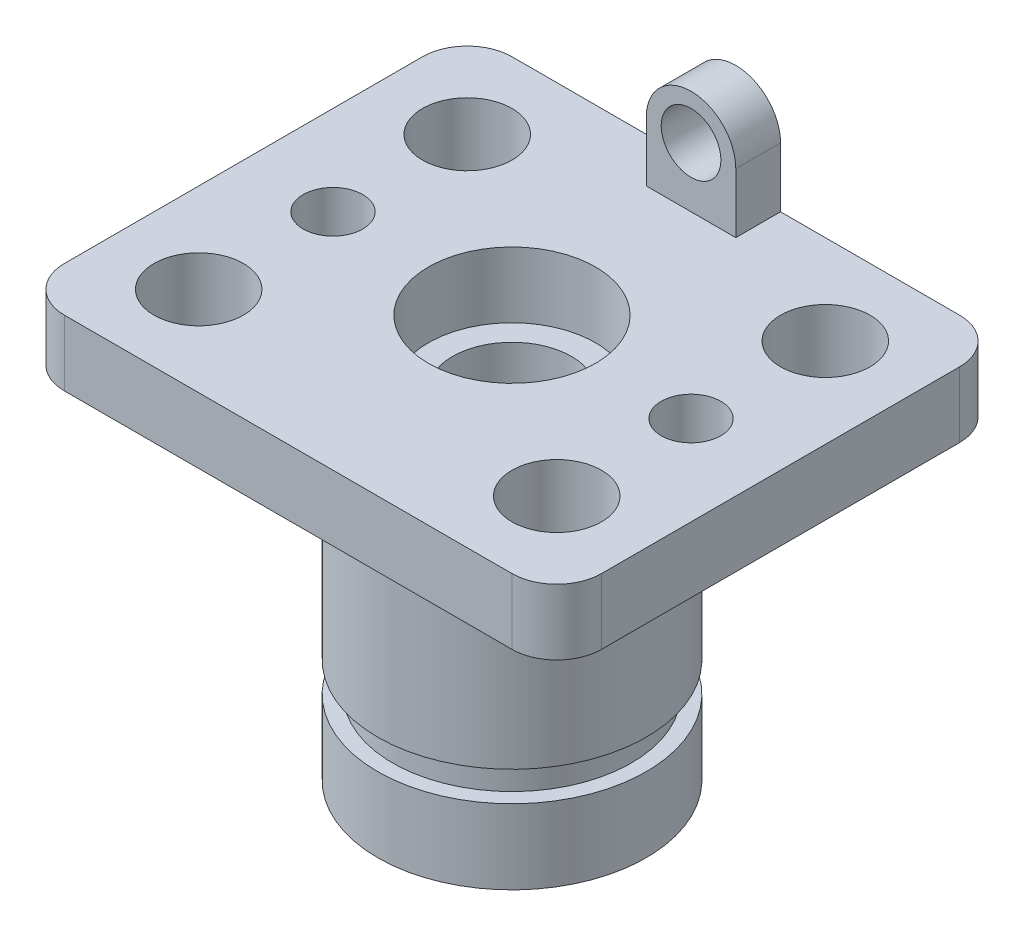
ISO-10303-21;
HEADER;
FILE_DESCRIPTION(('STEP AP214'),'2;1');
FILE_NAME('part.step','',(''),(''),'','','');
FILE_SCHEMA(('AUTOMOTIVE_DESIGN { 1 0 10303 214 1 1 1 1 }'));
ENDSEC;
DATA;
#1=APPLICATION_CONTEXT('core data for automotive mechanical design processes');
#2=APPLICATION_PROTOCOL_DEFINITION('international standard','automotive_design',2000,#1);
#3=PRODUCT_CONTEXT('',#1,'mechanical');
#4=PRODUCT('Part','Part','',(#3));
#5=PRODUCT_RELATED_PRODUCT_CATEGORY('part','',(#4));
#6=PRODUCT_DEFINITION_FORMATION('','',#4);
#7=PRODUCT_DEFINITION_CONTEXT('part definition',#1,'design');
#8=PRODUCT_DEFINITION('design','',#6,#7);
#9=PRODUCT_DEFINITION_SHAPE('','',#8);
#10=(LENGTH_UNIT() NAMED_UNIT(*) SI_UNIT(.MILLI.,.METRE.));
#11=(NAMED_UNIT(*) PLANE_ANGLE_UNIT() SI_UNIT($,.RADIAN.));
#12=(NAMED_UNIT(*) SI_UNIT($,.STERADIAN.) SOLID_ANGLE_UNIT());
#13=UNCERTAINTY_MEASURE_WITH_UNIT(LENGTH_MEASURE(1.E-05),#10,'distance_accuracy_value','');
#14=(GEOMETRIC_REPRESENTATION_CONTEXT(3) GLOBAL_UNCERTAINTY_ASSIGNED_CONTEXT((#13)) GLOBAL_UNIT_ASSIGNED_CONTEXT((#10,
#11,#12)) REPRESENTATION_CONTEXT('',''));
#15=CARTESIAN_POINT('',(0.,0.,0.));
#16=DIRECTION('',(0.,0.,1.));
#17=DIRECTION('',(1.,0.,0.));
#18=AXIS2_PLACEMENT_3D('',#15,#16,#17);
#19=CARTESIAN_POINT('',(-28000.,135000.,0.));
#20=DIRECTION('',(0.,-1.,0.));
#21=DIRECTION('',(0.,0.,-1.));
#22=AXIS2_PLACEMENT_3D('',#19,#20,#21);
#23=PLANE('',#22);
#24=CARTESIAN_POINT('',(0.,135000.,0.));
#25=DIRECTION('',(0.,1.,0.));
#26=DIRECTION('',(0.,0.,1.));
#27=AXIS2_PLACEMENT_3D('',#24,#25,#26);
#28=CIRCLE('',#27,28000.);
#29=CARTESIAN_POINT('',(0.,135000.,28000.));
#30=VERTEX_POINT('',#29);
#31=EDGE_CURVE('E200',#30,#30,#28,.T.);
#32=ORIENTED_EDGE('',*,*,#31,.F.);
#33=EDGE_LOOP('',(#32));
#34=FACE_BOUND('',#33,.T.);
#35=CARTESIAN_POINT('',(-60000.,135000.,45000.));
#36=DIRECTION('',(0.,1.,0.));
#37=DIRECTION('',(0.,0.,1.));
#38=AXIS2_PLACEMENT_3D('',#35,#36,#37);
#39=CIRCLE('',#38,15000.);
#40=CARTESIAN_POINT('',(-60000.,135000.,60000.));
#41=VERTEX_POINT('',#40);
#42=EDGE_CURVE('E195',#41,#41,#39,.T.);
#43=ORIENTED_EDGE('',*,*,#42,.F.);
#44=EDGE_LOOP('',(#43));
#45=FACE_BOUND('',#44,.T.);
#46=CARTESIAN_POINT('',(-60000.,135000.,0.));
#47=DIRECTION('',(0.,1.,0.));
#48=DIRECTION('',(0.,0.,1.));
#49=AXIS2_PLACEMENT_3D('',#46,#47,#48);
#50=CIRCLE('',#49,10000.);
#51=CARTESIAN_POINT('',(-60000.,135000.,10000.));
#52=VERTEX_POINT('',#51);
#53=EDGE_CURVE('E187',#52,#52,#50,.T.);
#54=ORIENTED_EDGE('',*,*,#53,.F.);
#55=EDGE_LOOP('',(#54));
#56=FACE_BOUND('',#55,.T.);
#57=CARTESIAN_POINT('',(-60000.,135000.,-45000.));
#58=DIRECTION('',(0.,1.,0.));
#59=DIRECTION('',(0.,0.,1.));
#60=AXIS2_PLACEMENT_3D('',#57,#58,#59);
#61=CIRCLE('',#60,15000.);
#62=CARTESIAN_POINT('',(-60000.,135000.,-30000.));
#63=VERTEX_POINT('',#62);
#64=EDGE_CURVE('E190',#63,#63,#61,.T.);
#65=ORIENTED_EDGE('',*,*,#64,.F.);
#66=EDGE_LOOP('',(#65));
#67=FACE_BOUND('',#66,.T.);
#68=CARTESIAN_POINT('',(60000.0000000001,135000.,-45000.));
#69=DIRECTION('',(0.,-1.,0.));
#70=DIRECTION('',(0.,0.,-1.));
#71=AXIS2_PLACEMENT_3D('',#68,#69,#70);
#72=CIRCLE('',#71,15000.);
#73=CARTESIAN_POINT('',(60000.0000000001,135000.,-60000.));
#74=VERTEX_POINT('',#73);
#75=EDGE_CURVE('E44',#74,#74,#72,.F.);
#76=ORIENTED_EDGE('',*,*,#75,.F.);
#77=EDGE_LOOP('',(#76));
#78=FACE_BOUND('',#77,.T.);
#79=CARTESIAN_POINT('',(60000.0000000001,135000.,0.));
#80=DIRECTION('',(0.,1.,0.));
#81=DIRECTION('',(0.,0.,1.));
#82=AXIS2_PLACEMENT_3D('',#79,#80,#81);
#83=CIRCLE('',#82,10000.);
#84=CARTESIAN_POINT('',(60000.0000000001,135000.,10000.));
#85=VERTEX_POINT('',#84);
#86=EDGE_CURVE('E172',#85,#85,#83,.T.);
#87=ORIENTED_EDGE('',*,*,#86,.F.);
#88=EDGE_LOOP('',(#87));
#89=FACE_BOUND('',#88,.T.);
#90=CARTESIAN_POINT('',(60000.0000000001,135000.,45000.));
#91=DIRECTION('',(0.,1.,0.));
#92=DIRECTION('',(0.,0.,1.));
#93=AXIS2_PLACEMENT_3D('',#90,#91,#92);
#94=CIRCLE('',#93,15000.);
#95=CARTESIAN_POINT('',(60000.0000000001,135000.,60000.));
#96=VERTEX_POINT('',#95);
#97=EDGE_CURVE('E164',#96,#96,#94,.T.);
#98=ORIENTED_EDGE('',*,*,#97,.F.);
#99=EDGE_LOOP('',(#98));
#100=FACE_BOUND('',#99,.T.);
#101=DIRECTION('',(0.,0.,-1.));
#102=VECTOR('',#101,1.);
#103=CARTESIAN_POINT('',(15000.,135000.,-60000.));
#104=LINE('',#103,#102);
#105=CARTESIAN_POINT('',(15000.,135000.,-60000.));
#106=VERTEX_POINT('',#105);
#107=CARTESIAN_POINT('',(15000.,135000.,-75000.));
#108=VERTEX_POINT('',#107);
#109=EDGE_CURVE('E148',#106,#108,#104,.T.);
#110=ORIENTED_EDGE('',*,*,#109,.F.);
#111=DIRECTION('',(-1.,0.,0.));
#112=VECTOR('',#111,1.);
#113=CARTESIAN_POINT('',(15000.,135000.,-60000.));
#114=LINE('',#113,#112);
#115=CARTESIAN_POINT('',(-15000.,135000.,-60000.));
#116=VERTEX_POINT('',#115);
#117=EDGE_CURVE('E145',#106,#116,#114,.T.);
#118=ORIENTED_EDGE('',*,*,#117,.T.);
#119=DIRECTION('',(0.,0.,-1.));
#120=VECTOR('',#119,1.);
#121=CARTESIAN_POINT('',(-15000.,135000.,-60000.));
#122=LINE('',#121,#120);
#123=CARTESIAN_POINT('',(-15000.,135000.,-75000.));
#124=VERTEX_POINT('',#123);
#125=EDGE_CURVE('E130',#116,#124,#122,.T.);
#126=ORIENTED_EDGE('',*,*,#125,.T.);
#127=DIRECTION('',(-1.,0.,0.));
#128=VECTOR('',#127,1.);
#129=CARTESIAN_POINT('',(-90000.,135000.,-75000.));
#130=LINE('',#129,#128);
#131=CARTESIAN_POINT('',(-75000.,135000.,-75000.));
#132=VERTEX_POINT('',#131);
#133=EDGE_CURVE('E225',#124,#132,#130,.T.);
#134=ORIENTED_EDGE('',*,*,#133,.T.);
#135=CARTESIAN_POINT('',(-75000.,135000.,-60000.));
#136=DIRECTION('',(0.,-1.,0.));
#137=DIRECTION('',(0.,0.,-1.));
#138=AXIS2_PLACEMENT_3D('',#135,#136,#137);
#139=CIRCLE('',#138,15000.);
#140=CARTESIAN_POINT('',(-90000.,135000.,-60000.));
#141=VERTEX_POINT('',#140);
#142=EDGE_CURVE('E271',#132,#141,#139,.F.);
#143=ORIENTED_EDGE('',*,*,#142,.T.);
#144=DIRECTION('',(0.,0.,1.));
#145=VECTOR('',#144,1.);
#146=CARTESIAN_POINT('',(-90000.,135000.,-75000.));
#147=LINE('',#146,#145);
#148=CARTESIAN_POINT('',(-89999.9999999999,135000.,60000.));
#149=VERTEX_POINT('',#148);
#150=EDGE_CURVE('E221',#141,#149,#147,.T.);
#151=ORIENTED_EDGE('',*,*,#150,.T.);
#152=CARTESIAN_POINT('',(-74999.9999999999,135000.,60000.));
#153=DIRECTION('',(0.,-1.,0.));
#154=DIRECTION('',(0.,0.,-1.));
#155=AXIS2_PLACEMENT_3D('',#152,#153,#154);
#156=CIRCLE('',#155,15000.);
#157=CARTESIAN_POINT('',(-74999.9999999999,135000.,75000.));
#158=VERTEX_POINT('',#157);
#159=EDGE_CURVE('E262',#149,#158,#156,.F.);
#160=ORIENTED_EDGE('',*,*,#159,.T.);
#161=DIRECTION('',(1.,0.,0.));
#162=VECTOR('',#161,1.);
#163=CARTESIAN_POINT('',(-89999.9999999999,135000.,75000.));
#164=LINE('',#163,#162);
#165=CARTESIAN_POINT('',(75000.0000000001,135000.,75000.));
#166=VERTEX_POINT('',#165);
#167=EDGE_CURVE('E211',#158,#166,#164,.T.);
#168=ORIENTED_EDGE('',*,*,#167,.T.);
#169=CARTESIAN_POINT('',(75000.0000000001,135000.,60000.));
#170=DIRECTION('',(0.,-1.,0.));
#171=DIRECTION('',(0.,0.,-1.));
#172=AXIS2_PLACEMENT_3D('',#169,#170,#171);
#173=CIRCLE('',#172,15000.);
#174=CARTESIAN_POINT('',(90000.0000000001,135000.,60000.));
#175=VERTEX_POINT('',#174);
#176=EDGE_CURVE('E254',#166,#175,#173,.F.);
#177=ORIENTED_EDGE('',*,*,#176,.T.);
#178=DIRECTION('',(0.,0.,-1.));
#179=VECTOR('',#178,1.);
#180=CARTESIAN_POINT('',(90000.,135000.,-75000.));
#181=LINE('',#180,#179);
#182=CARTESIAN_POINT('',(90000.,135000.,-60000.));
#183=VERTEX_POINT('',#182);
#184=EDGE_CURVE('E220',#175,#183,#181,.T.);
#185=ORIENTED_EDGE('',*,*,#184,.T.);
#186=CARTESIAN_POINT('',(75000.,135000.,-60000.));
#187=DIRECTION('',(0.,-1.,0.));
#188=DIRECTION('',(0.,0.,-1.));
#189=AXIS2_PLACEMENT_3D('',#186,#187,#188);
#190=CIRCLE('',#189,15000.);
#191=CARTESIAN_POINT('',(75000.,135000.,-75000.));
#192=VERTEX_POINT('',#191);
#193=EDGE_CURVE('E282',#183,#192,#190,.F.);
#194=ORIENTED_EDGE('',*,*,#193,.T.);
#195=EDGE_CURVE('E223',#192,#108,#130,.T.);
#196=ORIENTED_EDGE('',*,*,#195,.T.);
#197=EDGE_LOOP('',(#110,#118,#126,#134,#143,#151,#160,#168,#177,#185,#194,#196));
#198=FACE_BOUND('',#197,.T.);
#199=ADVANCED_FACE('F41',(#34,#45,#56,#67,#78,#89,#100,#198),#23,.F.);
#200=CARTESIAN_POINT('',(0.,0.,0.));
#201=DIRECTION('',(0.,-1.,0.));
#202=DIRECTION('',(0.,0.,-1.));
#203=AXIS2_PLACEMENT_3D('',#200,#201,#202);
#204=CYLINDRICAL_SURFACE('',#203,20000.);
#205=CARTESIAN_POINT('',(0.,0.,0.));
#206=DIRECTION('',(0.,-1.,0.));
#207=DIRECTION('',(0.,0.,-1.));
#208=AXIS2_PLACEMENT_3D('',#205,#206,#207);
#209=CIRCLE('',#208,20000.);
#210=CARTESIAN_POINT('',(0.,0.,-20000.));
#211=VERTEX_POINT('',#210);
#212=EDGE_CURVE('E242',#211,#211,#209,.T.);
#213=ORIENTED_EDGE('',*,*,#212,.T.);
#214=EDGE_LOOP('',(#213));
#215=FACE_BOUND('',#214,.T.);
#216=CARTESIAN_POINT('',(0.,113000.,0.));
#217=DIRECTION('',(0.,1.,0.));
#218=DIRECTION('',(0.,0.,1.));
#219=AXIS2_PLACEMENT_3D('',#216,#217,#218);
#220=CIRCLE('',#219,20000.);
#221=CARTESIAN_POINT('',(0.,113000.,20000.));
#222=VERTEX_POINT('',#221);
#223=EDGE_CURVE('E201',#222,#222,#220,.F.);
#224=ORIENTED_EDGE('',*,*,#223,.F.);
#225=EDGE_LOOP('',(#224));
#226=FACE_BOUND('',#225,.T.);
#227=ADVANCED_FACE('F331',(#215,#226),#204,.F.);
#228=CARTESIAN_POINT('',(0.,0.,0.));
#229=DIRECTION('',(0.,-1.,0.));
#230=DIRECTION('',(0.,0.,-1.));
#231=AXIS2_PLACEMENT_3D('',#228,#229,#230);
#232=CYLINDRICAL_SURFACE('',#231,45000.);
#233=CARTESIAN_POINT('',(0.,35000.,0.));
#234=DIRECTION('',(0.,-1.,0.));
#235=DIRECTION('',(0.,0.,-1.));
#236=AXIS2_PLACEMENT_3D('',#233,#234,#235);
#237=CIRCLE('',#236,45000.);
#238=CARTESIAN_POINT('',(0.,35000.,-45000.));
#239=VERTEX_POINT('',#238);
#240=EDGE_CURVE('E241',#239,#239,#237,.T.);
#241=ORIENTED_EDGE('',*,*,#240,.F.);
#242=EDGE_LOOP('',(#241));
#243=FACE_BOUND('',#242,.T.);
#244=CARTESIAN_POINT('',(0.,113000.,0.));
#245=DIRECTION('',(0.,1.,0.));
#246=DIRECTION('',(0.,0.,1.));
#247=AXIS2_PLACEMENT_3D('',#244,#245,#246);
#248=CIRCLE('',#247,45000.);
#249=CARTESIAN_POINT('',(0.,113000.,45000.));
#250=VERTEX_POINT('',#249);
#251=EDGE_CURVE('E250',#250,#250,#248,.T.);
#252=ORIENTED_EDGE('',*,*,#251,.F.);
#253=EDGE_LOOP('',(#252));
#254=FACE_BOUND('',#253,.T.);
#255=ADVANCED_FACE('F345',(#243,#254),#232,.T.);
#256=CARTESIAN_POINT('',(-45000.,-2.36390366877063E-12,0.));
#257=DIRECTION('',(0.,1.,0.));
#258=DIRECTION('',(0.,0.,1.));
#259=AXIS2_PLACEMENT_3D('',#256,#257,#258);
#260=PLANE('',#259);
#261=ORIENTED_EDGE('',*,*,#212,.F.);
#262=EDGE_LOOP('',(#261));
#263=FACE_BOUND('',#262,.T.);
#264=CARTESIAN_POINT('',(0.,-4.72780733754125E-12,0.));
#265=DIRECTION('',(0.,-1.,0.));
#266=DIRECTION('',(0.,0.,-1.));
#267=AXIS2_PLACEMENT_3D('',#264,#265,#266);
#268=CIRCLE('',#267,45000.);
#269=CARTESIAN_POINT('',(0.,-4.72780733754125E-12,-45000.));
#270=VERTEX_POINT('',#269);
#271=EDGE_CURVE('E217',#270,#270,#268,.T.);
#272=ORIENTED_EDGE('',*,*,#271,.T.);
#273=EDGE_LOOP('',(#272));
#274=FACE_BOUND('',#273,.T.);
#275=ADVANCED_FACE('F352',(#263,#274),#260,.F.);
#276=CARTESIAN_POINT('',(-45000.,35000.,0.));
#277=DIRECTION('',(0.,1.,0.));
#278=DIRECTION('',(0.,0.,1.));
#279=AXIS2_PLACEMENT_3D('',#276,#277,#278);
#280=PLANE('',#279);
#281=CARTESIAN_POINT('',(0.,35000.,0.));
#282=DIRECTION('',(0.,-1.,0.));
#283=DIRECTION('',(0.,0.,-1.));
#284=AXIS2_PLACEMENT_3D('',#281,#282,#283);
#285=CIRCLE('',#284,40000.);
#286=CARTESIAN_POINT('',(0.,35000.,-40000.));
#287=VERTEX_POINT('',#286);
#288=EDGE_CURVE('E238',#287,#287,#285,.T.);
#289=ORIENTED_EDGE('',*,*,#288,.F.);
#290=EDGE_LOOP('',(#289));
#291=FACE_BOUND('',#290,.T.);
#292=ORIENTED_EDGE('',*,*,#240,.T.);
#293=EDGE_LOOP('',(#292));
#294=FACE_BOUND('',#293,.T.);
#295=ADVANCED_FACE('F354',(#291,#294),#280,.F.);
#296=CARTESIAN_POINT('',(0.,0.,0.));
#297=DIRECTION('',(0.,-1.,0.));
#298=DIRECTION('',(0.,0.,-1.));
#299=AXIS2_PLACEMENT_3D('',#296,#297,#298);
#300=CYLINDRICAL_SURFACE('',#299,40000.);
#301=CARTESIAN_POINT('',(0.,25000.,0.));
#302=DIRECTION('',(0.,-1.,0.));
#303=DIRECTION('',(0.,0.,-1.));
#304=AXIS2_PLACEMENT_3D('',#301,#302,#303);
#305=CIRCLE('',#304,40000.);
#306=CARTESIAN_POINT('',(0.,25000.,-40000.));
#307=VERTEX_POINT('',#306);
#308=EDGE_CURVE('E232',#307,#307,#305,.T.);
#309=ORIENTED_EDGE('',*,*,#308,.F.);
#310=EDGE_LOOP('',(#309));
#311=FACE_BOUND('',#310,.T.);
#312=ORIENTED_EDGE('',*,*,#288,.T.);
#313=EDGE_LOOP('',(#312));
#314=FACE_BOUND('',#313,.T.);
#315=ADVANCED_FACE('F420',(#311,#314),#300,.T.);
#316=CARTESIAN_POINT('',(-40000.,25000.,0.));
#317=DIRECTION('',(0.,-1.,0.));
#318=DIRECTION('',(0.,0.,-1.));
#319=AXIS2_PLACEMENT_3D('',#316,#317,#318);
#320=PLANE('',#319);
#321=CARTESIAN_POINT('',(0.,25000.,0.));
#322=DIRECTION('',(0.,-1.,0.));
#323=DIRECTION('',(0.,0.,-1.));
#324=AXIS2_PLACEMENT_3D('',#321,#322,#323);
#325=CIRCLE('',#324,45000.);
#326=CARTESIAN_POINT('',(0.,25000.,-45000.));
#327=VERTEX_POINT('',#326);
#328=EDGE_CURVE('E235',#327,#327,#325,.T.);
#329=ORIENTED_EDGE('',*,*,#328,.F.);
#330=EDGE_LOOP('',(#329));
#331=FACE_BOUND('',#330,.T.);
#332=ORIENTED_EDGE('',*,*,#308,.T.);
#333=EDGE_LOOP('',(#332));
#334=FACE_BOUND('',#333,.T.);
#335=ADVANCED_FACE('F395',(#331,#334),#320,.F.);
#336=CARTESIAN_POINT('',(0.,0.,0.));
#337=DIRECTION('',(0.,-1.,0.));
#338=DIRECTION('',(0.,0.,-1.));
#339=AXIS2_PLACEMENT_3D('',#336,#337,#338);
#340=CYLINDRICAL_SURFACE('',#339,45000.);
#341=ORIENTED_EDGE('',*,*,#271,.F.);
#342=EDGE_LOOP('',(#341));
#343=FACE_BOUND('',#342,.T.);
#344=ORIENTED_EDGE('',*,*,#328,.T.);
#345=EDGE_LOOP('',(#344));
#346=FACE_BOUND('',#345,.T.);
#347=ADVANCED_FACE('F383',(#343,#346),#340,.T.);
#348=CARTESIAN_POINT('',(0.,113000.,0.));
#349=DIRECTION('',(0.,1.,0.));
#350=DIRECTION('',(0.,0.,1.));
#351=AXIS2_PLACEMENT_3D('',#348,#349,#350);
#352=PLANE('',#351);
#353=CARTESIAN_POINT('',(60000.0000000001,113000.,45000.));
#354=DIRECTION('',(0.,1.,0.));
#355=DIRECTION('',(0.,0.,1.));
#356=AXIS2_PLACEMENT_3D('',#353,#354,#355);
#357=CIRCLE('',#356,15000.);
#358=CARTESIAN_POINT('',(60000.0000000001,113000.,60000.));
#359=VERTEX_POINT('',#358);
#360=EDGE_CURVE('E171',#359,#359,#357,.F.);
#361=ORIENTED_EDGE('',*,*,#360,.F.);
#362=EDGE_LOOP('',(#361));
#363=FACE_BOUND('',#362,.T.);
#364=CARTESIAN_POINT('',(60000.0000000001,113000.,0.));
#365=DIRECTION('',(0.,1.,0.));
#366=DIRECTION('',(0.,0.,1.));
#367=AXIS2_PLACEMENT_3D('',#364,#365,#366);
#368=CIRCLE('',#367,10000.);
#369=CARTESIAN_POINT('',(60000.0000000001,113000.,10000.));
#370=VERTEX_POINT('',#369);
#371=EDGE_CURVE('E180',#370,#370,#368,.F.);
#372=ORIENTED_EDGE('',*,*,#371,.F.);
#373=EDGE_LOOP('',(#372));
#374=FACE_BOUND('',#373,.T.);
#375=CARTESIAN_POINT('',(60000.0000000001,113000.,-45000.));
#376=DIRECTION('',(0.,1.,0.));
#377=DIRECTION('',(0.,0.,1.));
#378=AXIS2_PLACEMENT_3D('',#375,#376,#377);
#379=CIRCLE('',#378,15000.);
#380=CARTESIAN_POINT('',(60000.0000000001,113000.,-60000.));
#381=VERTEX_POINT('',#380);
#382=EDGE_CURVE('E179',#381,#381,#379,.F.);
#383=ORIENTED_EDGE('',*,*,#382,.F.);
#384=EDGE_LOOP('',(#383));
#385=FACE_BOUND('',#384,.T.);
#386=CARTESIAN_POINT('',(-60000.,113000.,-45000.));
#387=DIRECTION('',(0.,1.,0.));
#388=DIRECTION('',(0.,0.,1.));
#389=AXIS2_PLACEMENT_3D('',#386,#387,#388);
#390=CIRCLE('',#389,15000.);
#391=CARTESIAN_POINT('',(-60000.,113000.,-30000.));
#392=VERTEX_POINT('',#391);
#393=EDGE_CURVE('E182',#392,#392,#390,.T.);
#394=ORIENTED_EDGE('',*,*,#393,.T.);
#395=EDGE_LOOP('',(#394));
#396=FACE_BOUND('',#395,.T.);
#397=CARTESIAN_POINT('',(-60000.,113000.,0.));
#398=DIRECTION('',(0.,1.,0.));
#399=DIRECTION('',(0.,0.,1.));
#400=AXIS2_PLACEMENT_3D('',#397,#398,#399);
#401=CIRCLE('',#400,10000.);
#402=CARTESIAN_POINT('',(-60000.,113000.,10000.));
#403=VERTEX_POINT('',#402);
#404=EDGE_CURVE('E188',#403,#403,#401,.T.);
#405=ORIENTED_EDGE('',*,*,#404,.T.);
#406=EDGE_LOOP('',(#405));
#407=FACE_BOUND('',#406,.T.);
#408=CARTESIAN_POINT('',(-60000.,113000.,45000.));
#409=DIRECTION('',(0.,1.,0.));
#410=DIRECTION('',(0.,0.,1.));
#411=AXIS2_PLACEMENT_3D('',#408,#409,#410);
#412=CIRCLE('',#411,15000.);
#413=CARTESIAN_POINT('',(-60000.,113000.,60000.));
#414=VERTEX_POINT('',#413);
#415=EDGE_CURVE('E198',#414,#414,#412,.T.);
#416=ORIENTED_EDGE('',*,*,#415,.T.);
#417=EDGE_LOOP('',(#416));
#418=FACE_BOUND('',#417,.T.);
#419=ORIENTED_EDGE('',*,*,#251,.T.);
#420=EDGE_LOOP('',(#419));
#421=FACE_BOUND('',#420,.T.);
#422=DIRECTION('',(-1.,0.,0.));
#423=VECTOR('',#422,1.);
#424=CARTESIAN_POINT('',(-90000.,113000.,-75000.));
#425=LINE('',#424,#423);
#426=CARTESIAN_POINT('',(75000.,113000.,-75000.));
#427=VERTEX_POINT('',#426);
#428=CARTESIAN_POINT('',(-75000.,113000.,-75000.));
#429=VERTEX_POINT('',#428);
#430=EDGE_CURVE('E214',#427,#429,#425,.T.);
#431=ORIENTED_EDGE('',*,*,#430,.F.);
#432=CARTESIAN_POINT('',(75000.,113000.,-60000.));
#433=DIRECTION('',(0.,1.,0.));
#434=DIRECTION('',(0.,0.,1.));
#435=AXIS2_PLACEMENT_3D('',#432,#433,#434);
#436=CIRCLE('',#435,15000.);
#437=CARTESIAN_POINT('',(90000.,113000.,-60000.));
#438=VERTEX_POINT('',#437);
#439=EDGE_CURVE('E11',#427,#438,#436,.F.);
#440=ORIENTED_EDGE('',*,*,#439,.T.);
#441=DIRECTION('',(0.,0.,-1.));
#442=VECTOR('',#441,1.);
#443=CARTESIAN_POINT('',(90000.,113000.,-75000.));
#444=LINE('',#443,#442);
#445=CARTESIAN_POINT('',(90000.0000000001,113000.,60000.));
#446=VERTEX_POINT('',#445);
#447=EDGE_CURVE('E206',#446,#438,#444,.T.);
#448=ORIENTED_EDGE('',*,*,#447,.F.);
#449=CARTESIAN_POINT('',(75000.0000000001,113000.,60000.));
#450=DIRECTION('',(0.,1.,0.));
#451=DIRECTION('',(0.,0.,1.));
#452=AXIS2_PLACEMENT_3D('',#449,#450,#451);
#453=CIRCLE('',#452,15000.);
#454=CARTESIAN_POINT('',(75000.0000000001,113000.,75000.));
#455=VERTEX_POINT('',#454);
#456=EDGE_CURVE('E256',#446,#455,#453,.F.);
#457=ORIENTED_EDGE('',*,*,#456,.T.);
#458=DIRECTION('',(1.,0.,0.));
#459=VECTOR('',#458,1.);
#460=CARTESIAN_POINT('',(-89999.9999999999,113000.,75000.));
#461=LINE('',#460,#459);
#462=CARTESIAN_POINT('',(-74999.9999999999,113000.,75000.));
#463=VERTEX_POINT('',#462);
#464=EDGE_CURVE('E218',#463,#455,#461,.T.);
#465=ORIENTED_EDGE('',*,*,#464,.F.);
#466=CARTESIAN_POINT('',(-74999.9999999999,113000.,60000.));
#467=DIRECTION('',(0.,1.,0.));
#468=DIRECTION('',(0.,0.,1.));
#469=AXIS2_PLACEMENT_3D('',#466,#467,#468);
#470=CIRCLE('',#469,15000.);
#471=CARTESIAN_POINT('',(-89999.9999999999,113000.,60000.));
#472=VERTEX_POINT('',#471);
#473=EDGE_CURVE('E270',#463,#472,#470,.F.);
#474=ORIENTED_EDGE('',*,*,#473,.T.);
#475=DIRECTION('',(0.,0.,1.));
#476=VECTOR('',#475,1.);
#477=CARTESIAN_POINT('',(-90000.,113000.,-75000.));
#478=LINE('',#477,#476);
#479=CARTESIAN_POINT('',(-90000.,113000.,-60000.));
#480=VERTEX_POINT('',#479);
#481=EDGE_CURVE('E213',#480,#472,#478,.T.);
#482=ORIENTED_EDGE('',*,*,#481,.F.);
#483=CARTESIAN_POINT('',(-75000.,113000.,-60000.));
#484=DIRECTION('',(0.,1.,0.));
#485=DIRECTION('',(0.,0.,1.));
#486=AXIS2_PLACEMENT_3D('',#483,#484,#485);
#487=CIRCLE('',#486,15000.);
#488=EDGE_CURVE('E276',#480,#429,#487,.F.);
#489=ORIENTED_EDGE('',*,*,#488,.T.);
#490=EDGE_LOOP('',(#431,#440,#448,#457,#465,#474,#482,#489));
#491=FACE_BOUND('',#490,.T.);
#492=ADVANCED_FACE('F291',(#363,#374,#385,#396,#407,#418,#421,#491),#352,.F.);
#493=CARTESIAN_POINT('',(-90000.,113000.,-75000.));
#494=DIRECTION('',(0.,0.,-1.));
#495=DIRECTION('',(-1.,0.,0.));
#496=AXIS2_PLACEMENT_3D('',#493,#494,#495);
#497=PLANE('',#496);
#498=CARTESIAN_POINT('',(0.,155000.,-75000.));
#499=DIRECTION('',(0.,0.,-1.));
#500=DIRECTION('',(-1.,0.,0.));
#501=AXIS2_PLACEMENT_3D('',#498,#499,#500);
#502=CIRCLE('',#501,10000.);
#503=CARTESIAN_POINT('',(-10000.,155000.,-75000.));
#504=VERTEX_POINT('',#503);
#505=EDGE_CURVE('E605',#504,#504,#502,.T.);
#506=ORIENTED_EDGE('',*,*,#505,.F.);
#507=EDGE_LOOP('',(#506));
#508=FACE_BOUND('',#507,.T.);
#509=ORIENTED_EDGE('',*,*,#195,.F.);
#510=DIRECTION('',(0.,1.,0.));
#511=VECTOR('',#510,1.);
#512=CARTESIAN_POINT('',(75000.,113000.,-75000.));
#513=LINE('',#512,#511);
#514=EDGE_CURVE('E49',#192,#427,#513,.F.);
#515=ORIENTED_EDGE('',*,*,#514,.T.);
#516=ORIENTED_EDGE('',*,*,#430,.T.);
#517=DIRECTION('',(0.,1.,0.));
#518=VECTOR('',#517,1.);
#519=CARTESIAN_POINT('',(-75000.,113000.,-75000.));
#520=LINE('',#519,#518);
#521=EDGE_CURVE('E266',#429,#132,#520,.T.);
#522=ORIENTED_EDGE('',*,*,#521,.T.);
#523=ORIENTED_EDGE('',*,*,#133,.F.);
#524=DIRECTION('',(0.,1.,0.));
#525=VECTOR('',#524,1.);
#526=CARTESIAN_POINT('',(-15000.,135000.,-75000.));
#527=LINE('',#526,#525);
#528=CARTESIAN_POINT('',(-15000.,155000.,-75000.));
#529=VERTEX_POINT('',#528);
#530=EDGE_CURVE('E60',#124,#529,#527,.T.);
#531=ORIENTED_EDGE('',*,*,#530,.T.);
#532=CARTESIAN_POINT('',(0.,155000.,-75000.));
#533=DIRECTION('',(0.,0.,-1.));
#534=DIRECTION('',(-1.,0.,0.));
#535=AXIS2_PLACEMENT_3D('',#532,#533,#534);
#536=CIRCLE('',#535,15000.);
#537=CARTESIAN_POINT('',(15000.,155000.,-75000.));
#538=VERTEX_POINT('',#537);
#539=EDGE_CURVE('E152',#529,#538,#536,.T.);
#540=ORIENTED_EDGE('',*,*,#539,.T.);
#541=DIRECTION('',(0.,-1.,0.));
#542=VECTOR('',#541,1.);
#543=CARTESIAN_POINT('',(15000.,155000.,-75000.));
#544=LINE('',#543,#542);
#545=EDGE_CURVE('E147',#538,#108,#544,.T.);
#546=ORIENTED_EDGE('',*,*,#545,.T.);
#547=EDGE_LOOP('',(#509,#515,#516,#522,#523,#531,#540,#546));
#548=FACE_BOUND('',#547,.T.);
#549=ADVANCED_FACE('F288',(#508,#548),#497,.T.);
#550=CARTESIAN_POINT('',(-90000.,113000.,-75000.));
#551=DIRECTION('',(-1.,0.,0.));
#552=DIRECTION('',(0.,0.,1.));
#553=AXIS2_PLACEMENT_3D('',#550,#551,#552);
#554=PLANE('',#553);
#555=ORIENTED_EDGE('',*,*,#150,.F.);
#556=DIRECTION('',(0.,1.,0.));
#557=VECTOR('',#556,1.);
#558=CARTESIAN_POINT('',(-90000.,113000.,-60000.));
#559=LINE('',#558,#557);
#560=EDGE_CURVE('E273',#141,#480,#559,.F.);
#561=ORIENTED_EDGE('',*,*,#560,.T.);
#562=ORIENTED_EDGE('',*,*,#481,.T.);
#563=DIRECTION('',(0.,1.,0.));
#564=VECTOR('',#563,1.);
#565=CARTESIAN_POINT('',(-89999.9999999999,113000.,60000.));
#566=LINE('',#565,#564);
#567=EDGE_CURVE('E257',#472,#149,#566,.T.);
#568=ORIENTED_EDGE('',*,*,#567,.T.);
#569=EDGE_LOOP('',(#555,#561,#562,#568));
#570=FACE_BOUND('',#569,.T.);
#571=ADVANCED_FACE('F312',(#570),#554,.T.);
#572=CARTESIAN_POINT('',(-89999.9999999999,113000.,75000.));
#573=DIRECTION('',(0.,0.,1.));
#574=DIRECTION('',(1.,0.,0.));
#575=AXIS2_PLACEMENT_3D('',#572,#573,#574);
#576=PLANE('',#575);
#577=ORIENTED_EDGE('',*,*,#167,.F.);
#578=DIRECTION('',(0.,1.,0.));
#579=VECTOR('',#578,1.);
#580=CARTESIAN_POINT('',(-74999.9999999999,113000.,75000.));
#581=LINE('',#580,#579);
#582=EDGE_CURVE('E261',#158,#463,#581,.F.);
#583=ORIENTED_EDGE('',*,*,#582,.T.);
#584=ORIENTED_EDGE('',*,*,#464,.T.);
#585=DIRECTION('',(0.,1.,0.));
#586=VECTOR('',#585,1.);
#587=CARTESIAN_POINT('',(75000.0000000001,113000.,75000.));
#588=LINE('',#587,#586);
#589=EDGE_CURVE('E249',#455,#166,#588,.T.);
#590=ORIENTED_EDGE('',*,*,#589,.T.);
#591=EDGE_LOOP('',(#577,#583,#584,#590));
#592=FACE_BOUND('',#591,.T.);
#593=ADVANCED_FACE('F324',(#592),#576,.T.);
#594=CARTESIAN_POINT('',(90000.,113000.,-75000.));
#595=DIRECTION('',(1.,0.,0.));
#596=DIRECTION('',(0.,0.,-1.));
#597=AXIS2_PLACEMENT_3D('',#594,#595,#596);
#598=PLANE('',#597);
#599=ORIENTED_EDGE('',*,*,#447,.T.);
#600=DIRECTION('',(0.,1.,0.));
#601=VECTOR('',#600,1.);
#602=CARTESIAN_POINT('',(90000.,113000.,-60000.));
#603=LINE('',#602,#601);
#604=EDGE_CURVE('E277',#438,#183,#603,.T.);
#605=ORIENTED_EDGE('',*,*,#604,.T.);
#606=ORIENTED_EDGE('',*,*,#184,.F.);
#607=DIRECTION('',(0.,1.,0.));
#608=VECTOR('',#607,1.);
#609=CARTESIAN_POINT('',(90000.0000000001,113000.,60000.));
#610=LINE('',#609,#608);
#611=EDGE_CURVE('E253',#175,#446,#610,.F.);
#612=ORIENTED_EDGE('',*,*,#611,.T.);
#613=EDGE_LOOP('',(#599,#605,#606,#612));
#614=FACE_BOUND('',#613,.T.);
#615=ADVANCED_FACE('F298',(#614),#598,.T.);
#616=CARTESIAN_POINT('',(0.,113000.,0.));
#617=DIRECTION('',(0.,1.,0.));
#618=DIRECTION('',(0.,0.,1.));
#619=AXIS2_PLACEMENT_3D('',#616,#617,#618);
#620=PLANE('',#619);
#621=CARTESIAN_POINT('',(0.,113000.,0.));
#622=DIRECTION('',(0.,1.,0.));
#623=DIRECTION('',(0.,0.,1.));
#624=AXIS2_PLACEMENT_3D('',#621,#622,#623);
#625=CIRCLE('',#624,28000.);
#626=CARTESIAN_POINT('',(0.,113000.,28000.));
#627=VERTEX_POINT('',#626);
#628=EDGE_CURVE('E205',#627,#627,#625,.T.);
#629=ORIENTED_EDGE('',*,*,#628,.T.);
#630=EDGE_LOOP('',(#629));
#631=FACE_BOUND('',#630,.T.);
#632=ORIENTED_EDGE('',*,*,#223,.T.);
#633=EDGE_LOOP('',(#632));
#634=FACE_BOUND('',#633,.T.);
#635=ADVANCED_FACE('F330',(#631,#634),#620,.T.);
#636=CARTESIAN_POINT('',(0.,113000.,0.));
#637=DIRECTION('',(0.,1.,0.));
#638=DIRECTION('',(0.,0.,1.));
#639=AXIS2_PLACEMENT_3D('',#636,#637,#638);
#640=CYLINDRICAL_SURFACE('',#639,28000.);
#641=ORIENTED_EDGE('',*,*,#628,.F.);
#642=EDGE_LOOP('',(#641));
#643=FACE_BOUND('',#642,.T.);
#644=ORIENTED_EDGE('',*,*,#31,.T.);
#645=EDGE_LOOP('',(#644));
#646=FACE_BOUND('',#645,.T.);
#647=ADVANCED_FACE('F357',(#643,#646),#640,.F.);
#648=CARTESIAN_POINT('',(75000.0000000001,113000.,60000.));
#649=DIRECTION('',(0.,1.,0.));
#650=DIRECTION('',(0.,0.,1.));
#651=AXIS2_PLACEMENT_3D('',#648,#649,#650);
#652=CYLINDRICAL_SURFACE('',#651,15000.);
#653=ORIENTED_EDGE('',*,*,#456,.F.);
#654=ORIENTED_EDGE('',*,*,#611,.F.);
#655=ORIENTED_EDGE('',*,*,#176,.F.);
#656=ORIENTED_EDGE('',*,*,#589,.F.);
#657=EDGE_LOOP('',(#653,#654,#655,#656));
#658=FACE_BOUND('',#657,.T.);
#659=ADVANCED_FACE('F297',(#658),#652,.T.);
#660=CARTESIAN_POINT('',(-74999.9999999999,113000.,60000.));
#661=DIRECTION('',(0.,1.,0.));
#662=DIRECTION('',(0.,0.,1.));
#663=AXIS2_PLACEMENT_3D('',#660,#661,#662);
#664=CYLINDRICAL_SURFACE('',#663,15000.);
#665=ORIENTED_EDGE('',*,*,#473,.F.);
#666=ORIENTED_EDGE('',*,*,#582,.F.);
#667=ORIENTED_EDGE('',*,*,#159,.F.);
#668=ORIENTED_EDGE('',*,*,#567,.F.);
#669=EDGE_LOOP('',(#665,#666,#667,#668));
#670=FACE_BOUND('',#669,.T.);
#671=ADVANCED_FACE('F307',(#670),#664,.T.);
#672=CARTESIAN_POINT('',(-75000.,113000.,-60000.));
#673=DIRECTION('',(0.,1.,0.));
#674=DIRECTION('',(0.,0.,1.));
#675=AXIS2_PLACEMENT_3D('',#672,#673,#674);
#676=CYLINDRICAL_SURFACE('',#675,15000.);
#677=ORIENTED_EDGE('',*,*,#488,.F.);
#678=ORIENTED_EDGE('',*,*,#560,.F.);
#679=ORIENTED_EDGE('',*,*,#142,.F.);
#680=ORIENTED_EDGE('',*,*,#521,.F.);
#681=EDGE_LOOP('',(#677,#678,#679,#680));
#682=FACE_BOUND('',#681,.T.);
#683=ADVANCED_FACE('F319',(#682),#676,.T.);
#684=CARTESIAN_POINT('',(75000.,113000.,-60000.));
#685=DIRECTION('',(0.,1.,0.));
#686=DIRECTION('',(0.,0.,1.));
#687=AXIS2_PLACEMENT_3D('',#684,#685,#686);
#688=CYLINDRICAL_SURFACE('',#687,15000.);
#689=ORIENTED_EDGE('',*,*,#439,.F.);
#690=ORIENTED_EDGE('',*,*,#514,.F.);
#691=ORIENTED_EDGE('',*,*,#193,.F.);
#692=ORIENTED_EDGE('',*,*,#604,.F.);
#693=EDGE_LOOP('',(#689,#690,#691,#692));
#694=FACE_BOUND('',#693,.T.);
#695=ADVANCED_FACE('F43',(#694),#688,.T.);
#696=CARTESIAN_POINT('',(-60000.,113000.,45000.));
#697=DIRECTION('',(0.,1.,0.));
#698=DIRECTION('',(0.,0.,1.));
#699=AXIS2_PLACEMENT_3D('',#696,#697,#698);
#700=CYLINDRICAL_SURFACE('',#699,15000.);
#701=ORIENTED_EDGE('',*,*,#415,.F.);
#702=EDGE_LOOP('',(#701));
#703=FACE_BOUND('',#702,.T.);
#704=ORIENTED_EDGE('',*,*,#42,.T.);
#705=EDGE_LOOP('',(#704));
#706=FACE_BOUND('',#705,.T.);
#707=ADVANCED_FACE('F365',(#703,#706),#700,.F.);
#708=CARTESIAN_POINT('',(-60000.,113000.,0.));
#709=DIRECTION('',(0.,1.,0.));
#710=DIRECTION('',(0.,0.,1.));
#711=AXIS2_PLACEMENT_3D('',#708,#709,#710);
#712=CYLINDRICAL_SURFACE('',#711,10000.);
#713=ORIENTED_EDGE('',*,*,#404,.F.);
#714=EDGE_LOOP('',(#713));
#715=FACE_BOUND('',#714,.T.);
#716=ORIENTED_EDGE('',*,*,#53,.T.);
#717=EDGE_LOOP('',(#716));
#718=FACE_BOUND('',#717,.T.);
#719=ADVANCED_FACE('F366',(#715,#718),#712,.F.);
#720=CARTESIAN_POINT('',(-60000.,113000.,-45000.));
#721=DIRECTION('',(0.,1.,0.));
#722=DIRECTION('',(0.,0.,1.));
#723=AXIS2_PLACEMENT_3D('',#720,#721,#722);
#724=CYLINDRICAL_SURFACE('',#723,15000.);
#725=ORIENTED_EDGE('',*,*,#393,.F.);
#726=EDGE_LOOP('',(#725));
#727=FACE_BOUND('',#726,.T.);
#728=ORIENTED_EDGE('',*,*,#64,.T.);
#729=EDGE_LOOP('',(#728));
#730=FACE_BOUND('',#729,.T.);
#731=ADVANCED_FACE('F375',(#727,#730),#724,.F.);
#732=CARTESIAN_POINT('',(60000.0000000001,135000.000012,-45000.));
#733=DIRECTION('',(0.,-1.,0.));
#734=DIRECTION('',(0.,0.,-1.));
#735=AXIS2_PLACEMENT_3D('',#732,#733,#734);
#736=CYLINDRICAL_SURFACE('',#735,15000.);
#737=CARTESIAN_POINT('',(60000.0000000001,113000.,-60000.));
#738=CARTESIAN_POINT('',(60000.0000000001,113229.166666667,-60000.));
#739=CARTESIAN_POINT('',(60000.0000000001,113458.333333333,-60000.));
#740=CARTESIAN_POINT('',(60000.0000000001,113916.666666667,-60000.));
#741=CARTESIAN_POINT('',(60000.0000000001,114145.833333333,-60000.));
#742=CARTESIAN_POINT('',(60000.0000000001,114604.166666667,-60000.));
#743=CARTESIAN_POINT('',(60000.0000000001,114833.333333333,-60000.));
#744=CARTESIAN_POINT('',(60000.0000000001,115291.666666667,-60000.));
#745=CARTESIAN_POINT('',(60000.0000000001,115520.833333333,-60000.));
#746=CARTESIAN_POINT('',(60000.0000000001,115979.166666667,-60000.));
#747=CARTESIAN_POINT('',(60000.0000000001,116208.333333333,-60000.));
#748=CARTESIAN_POINT('',(60000.0000000001,116666.666666667,-60000.));
#749=CARTESIAN_POINT('',(60000.0000000001,116895.833333333,-60000.));
#750=CARTESIAN_POINT('',(60000.0000000001,117354.166666667,-60000.));
#751=CARTESIAN_POINT('',(60000.0000000001,117583.333333333,-60000.));
#752=CARTESIAN_POINT('',(60000.0000000001,118041.666666667,-60000.));
#753=CARTESIAN_POINT('',(60000.0000000001,118270.833333333,-60000.));
#754=CARTESIAN_POINT('',(60000.0000000001,118729.166666667,-60000.));
#755=CARTESIAN_POINT('',(60000.0000000001,118958.333333333,-60000.));
#756=CARTESIAN_POINT('',(60000.0000000001,119416.666666667,-60000.));
#757=CARTESIAN_POINT('',(60000.0000000001,119645.833333333,-60000.));
#758=CARTESIAN_POINT('',(60000.0000000001,120104.166666667,-60000.));
#759=CARTESIAN_POINT('',(60000.0000000001,120333.333333333,-60000.));
#760=CARTESIAN_POINT('',(60000.0000000001,120791.666666667,-60000.));
#761=CARTESIAN_POINT('',(60000.0000000001,121020.833333333,-60000.));
#762=CARTESIAN_POINT('',(60000.0000000001,121479.166666667,-60000.));
#763=CARTESIAN_POINT('',(60000.0000000001,121708.333333333,-60000.));
#764=CARTESIAN_POINT('',(60000.0000000001,122166.666666667,-60000.));
#765=CARTESIAN_POINT('',(60000.0000000001,122395.833333333,-60000.));
#766=CARTESIAN_POINT('',(60000.0000000001,122854.166666667,-60000.));
#767=CARTESIAN_POINT('',(60000.0000000001,123083.333333333,-60000.));
#768=CARTESIAN_POINT('',(60000.0000000001,123541.666666667,-60000.));
#769=CARTESIAN_POINT('',(60000.0000000001,123770.833333333,-60000.));
#770=CARTESIAN_POINT('',(60000.0000000001,124229.166666667,-60000.));
#771=CARTESIAN_POINT('',(60000.0000000001,124458.333333333,-60000.));
#772=CARTESIAN_POINT('',(60000.0000000001,124916.666666667,-60000.));
#773=CARTESIAN_POINT('',(60000.0000000001,125145.833333333,-60000.));
#774=CARTESIAN_POINT('',(60000.0000000001,125604.166666667,-60000.));
#775=CARTESIAN_POINT('',(60000.0000000001,125833.333333333,-60000.));
#776=CARTESIAN_POINT('',(60000.0000000001,126291.666666667,-60000.));
#777=CARTESIAN_POINT('',(60000.0000000001,126520.833333333,-60000.));
#778=CARTESIAN_POINT('',(60000.0000000001,126979.166666667,-60000.));
#779=CARTESIAN_POINT('',(60000.0000000001,127208.333333333,-60000.));
#780=CARTESIAN_POINT('',(60000.0000000001,127666.666666667,-60000.));
#781=CARTESIAN_POINT('',(60000.0000000001,127895.833333333,-60000.));
#782=CARTESIAN_POINT('',(60000.0000000001,128354.166666667,-60000.));
#783=CARTESIAN_POINT('',(60000.0000000001,128583.333333333,-60000.));
#784=CARTESIAN_POINT('',(60000.0000000001,129041.666666667,-60000.));
#785=CARTESIAN_POINT('',(60000.0000000001,129270.833333333,-60000.));
#786=CARTESIAN_POINT('',(60000.0000000001,129729.166666667,-60000.));
#787=CARTESIAN_POINT('',(60000.0000000001,129958.333333333,-60000.));
#788=CARTESIAN_POINT('',(60000.0000000001,130416.666666667,-60000.));
#789=CARTESIAN_POINT('',(60000.0000000001,130645.833333333,-60000.));
#790=CARTESIAN_POINT('',(60000.0000000001,131104.166666667,-60000.));
#791=CARTESIAN_POINT('',(60000.0000000001,131333.333333333,-60000.));
#792=CARTESIAN_POINT('',(60000.0000000001,131791.666666667,-60000.));
#793=CARTESIAN_POINT('',(60000.0000000001,132020.833333333,-60000.));
#794=CARTESIAN_POINT('',(60000.0000000001,132479.166666667,-60000.));
#795=CARTESIAN_POINT('',(60000.0000000001,132708.333333333,-60000.));
#796=CARTESIAN_POINT('',(60000.0000000001,133166.666666667,-60000.));
#797=CARTESIAN_POINT('',(60000.0000000001,133395.833333333,-60000.));
#798=CARTESIAN_POINT('',(60000.0000000001,133854.166666667,-60000.));
#799=CARTESIAN_POINT('',(60000.0000000001,134083.333333333,-60000.));
#800=CARTESIAN_POINT('',(60000.0000000001,134541.666666667,-60000.));
#801=CARTESIAN_POINT('',(60000.0000000001,134770.833333333,-60000.));
#802=CARTESIAN_POINT('',(60000.0000000001,135000.,-60000.));
#803=B_SPLINE_CURVE_WITH_KNOTS('',3,(#737,#738,#739,#740,#741,#742,#743,#744,#745,#746,#747,
#748,#749,#750,#751,#752,#753,#754,#755,#756,#757,#758,#759,#760,#761,#762,#763,#764,#765,#766,
#767,#768,#769,#770,#771,#772,#773,#774,#775,#776,#777,#778,#779,#780,#781,#782,#783,#784,#785,
#786,#787,#788,#789,#790,#791,#792,#793,#794,#795,#796,#797,#798,#799,#800,#801,#802),
.UNSPECIFIED.,.F.,.F.,(4,2,2,2,2,2,2,2,2,2,2,2,2,2,2,2,2,2,2,2,2,2,2,2,2,2,2,2,2,2,2,2,4),(0.,
687.5,1375.,2062.50000000001,2750.00000000001,3437.50000000001,4125.00000000001,
4812.50000000001,5500.00000000001,6187.50000000001,6875.00000000001,7562.50000000001,
8250.00000000001,8937.50000000001,9625.00000000001,10312.5,11000.,11687.5,12375.,13062.5,13750.,
14437.5,15125.,15812.5,16500.,17187.5,17875.,18562.5,19250.,19937.5,20625.,21312.5,22000.),.UNSPECIFIED.);
#804=EDGE_CURVE('BSEAM518',#381,#74,#803,.T.);
#805=ORIENTED_EDGE('',*,*,#382,.T.);
#806=ORIENTED_EDGE('',*,*,#75,.T.);
#807=ORIENTED_EDGE('',*,*,#804,.T.);
#808=ORIENTED_EDGE('',*,*,#804,.F.);
#809=EDGE_LOOP('',(#805,#807,#806,#808));
#810=FACE_BOUND('',#809,.T.);
#811=ADVANCED_FACE('F518',(#810),#736,.F.);
#812=CARTESIAN_POINT('',(60000.0000000001,-0.000999999997475243,0.));
#813=DIRECTION('',(0.,1.,0.));
#814=DIRECTION('',(0.,0.,1.));
#815=AXIS2_PLACEMENT_3D('',#812,#813,#814);
#816=CYLINDRICAL_SURFACE('',#815,10000.);
#817=ORIENTED_EDGE('',*,*,#86,.T.);
#818=EDGE_LOOP('',(#817));
#819=FACE_BOUND('',#818,.T.);
#820=ORIENTED_EDGE('',*,*,#371,.T.);
#821=EDGE_LOOP('',(#820));
#822=FACE_BOUND('',#821,.T.);
#823=ADVANCED_FACE('F530',(#819,#822),#816,.F.);
#824=CARTESIAN_POINT('',(60000.0000000001,-0.000999999997475243,45000.));
#825=DIRECTION('',(0.,1.,0.));
#826=DIRECTION('',(0.,0.,1.));
#827=AXIS2_PLACEMENT_3D('',#824,#825,#826);
#828=CYLINDRICAL_SURFACE('',#827,15000.);
#829=ORIENTED_EDGE('',*,*,#97,.T.);
#830=EDGE_LOOP('',(#829));
#831=FACE_BOUND('',#830,.T.);
#832=ORIENTED_EDGE('',*,*,#360,.T.);
#833=EDGE_LOOP('',(#832));
#834=FACE_BOUND('',#833,.T.);
#835=ADVANCED_FACE('F533',(#831,#834),#828,.F.);
#836=CARTESIAN_POINT('',(15000.,155000.,-60000.));
#837=DIRECTION('',(1.,0.,0.));
#838=DIRECTION('',(0.,1.,0.));
#839=AXIS2_PLACEMENT_3D('',#836,#837,#838);
#840=PLANE('',#839);
#841=ORIENTED_EDGE('',*,*,#545,.F.);
#842=DIRECTION('',(0.,0.,-1.));
#843=VECTOR('',#842,1.);
#844=CARTESIAN_POINT('',(15000.,155000.,-60000.));
#845=LINE('',#844,#843);
#846=CARTESIAN_POINT('',(15000.,155000.,-60000.));
#847=VERTEX_POINT('',#846);
#848=EDGE_CURVE('E168',#847,#538,#845,.T.);
#849=ORIENTED_EDGE('',*,*,#848,.F.);
#850=DIRECTION('',(0.,-1.,0.));
#851=VECTOR('',#850,1.);
#852=CARTESIAN_POINT('',(15000.,155000.,-60000.));
#853=LINE('',#852,#851);
#854=EDGE_CURVE('E137',#847,#106,#853,.T.);
#855=ORIENTED_EDGE('',*,*,#854,.T.);
#856=ORIENTED_EDGE('',*,*,#109,.T.);
#857=EDGE_LOOP('',(#841,#849,#855,#856));
#858=FACE_BOUND('',#857,.T.);
#859=ADVANCED_FACE('F544',(#858),#840,.T.);
#860=CARTESIAN_POINT('',(0.,155000.,-60000.));
#861=DIRECTION('',(0.,0.,-1.));
#862=DIRECTION('',(-1.,0.,0.));
#863=AXIS2_PLACEMENT_3D('',#860,#861,#862);
#864=CYLINDRICAL_SURFACE('',#863,15000.);
#865=ORIENTED_EDGE('',*,*,#539,.F.);
#866=DIRECTION('',(0.,0.,-1.));
#867=VECTOR('',#866,1.);
#868=CARTESIAN_POINT('',(-15000.,155000.,-60000.));
#869=LINE('',#868,#867);
#870=CARTESIAN_POINT('',(-15000.,155000.,-60000.));
#871=VERTEX_POINT('',#870);
#872=EDGE_CURVE('E131',#871,#529,#869,.T.);
#873=ORIENTED_EDGE('',*,*,#872,.F.);
#874=CARTESIAN_POINT('',(0.,155000.,-60000.));
#875=DIRECTION('',(0.,0.,-1.));
#876=DIRECTION('',(-1.,0.,0.));
#877=AXIS2_PLACEMENT_3D('',#874,#875,#876);
#878=CIRCLE('',#877,15000.);
#879=EDGE_CURVE('E143',#871,#847,#878,.T.);
#880=ORIENTED_EDGE('',*,*,#879,.T.);
#881=ORIENTED_EDGE('',*,*,#848,.T.);
#882=EDGE_LOOP('',(#865,#873,#880,#881));
#883=FACE_BOUND('',#882,.T.);
#884=ADVANCED_FACE('F558',(#883),#864,.T.);
#885=CARTESIAN_POINT('',(-15000.,135000.,-60000.));
#886=DIRECTION('',(-1.,0.,0.));
#887=DIRECTION('',(0.,0.,1.));
#888=AXIS2_PLACEMENT_3D('',#885,#886,#887);
#889=PLANE('',#888);
#890=ORIENTED_EDGE('',*,*,#530,.F.);
#891=ORIENTED_EDGE('',*,*,#125,.F.);
#892=DIRECTION('',(0.,1.,0.));
#893=VECTOR('',#892,1.);
#894=CARTESIAN_POINT('',(-15000.,135000.,-60000.));
#895=LINE('',#894,#893);
#896=EDGE_CURVE('E133',#116,#871,#895,.T.);
#897=ORIENTED_EDGE('',*,*,#896,.T.);
#898=ORIENTED_EDGE('',*,*,#872,.T.);
#899=EDGE_LOOP('',(#890,#891,#897,#898));
#900=FACE_BOUND('',#899,.T.);
#901=ADVANCED_FACE('F127',(#900),#889,.T.);
#902=CARTESIAN_POINT('',(0.,155000.,-60000.));
#903=DIRECTION('',(0.,0.,-1.));
#904=DIRECTION('',(-1.,0.,0.));
#905=AXIS2_PLACEMENT_3D('',#902,#903,#904);
#906=PLANE('',#905);
#907=CARTESIAN_POINT('',(0.,155000.,-60000.));
#908=DIRECTION('',(0.,0.,-1.));
#909=DIRECTION('',(-1.,0.,0.));
#910=AXIS2_PLACEMENT_3D('',#907,#908,#909);
#911=CIRCLE('',#910,10000.);
#912=CARTESIAN_POINT('',(-10000.,155000.,-60000.));
#913=VERTEX_POINT('',#912);
#914=EDGE_CURVE('E157',#913,#913,#911,.F.);
#915=ORIENTED_EDGE('',*,*,#914,.F.);
#916=EDGE_LOOP('',(#915));
#917=FACE_BOUND('',#916,.T.);
#918=ORIENTED_EDGE('',*,*,#117,.F.);
#919=ORIENTED_EDGE('',*,*,#854,.F.);
#920=ORIENTED_EDGE('',*,*,#879,.F.);
#921=ORIENTED_EDGE('',*,*,#896,.F.);
#922=EDGE_LOOP('',(#918,#919,#920,#921));
#923=FACE_BOUND('',#922,.T.);
#924=ADVANCED_FACE('F136',(#917,#923),#906,.F.);
#925=CARTESIAN_POINT('',(0.,155000.,75000.001));
#926=DIRECTION('',(0.,0.,-1.));
#927=DIRECTION('',(-1.,0.,0.));
#928=AXIS2_PLACEMENT_3D('',#925,#926,#927);
#929=CYLINDRICAL_SURFACE('',#928,10000.);
#930=ORIENTED_EDGE('',*,*,#505,.T.);
#931=EDGE_LOOP('',(#930));
#932=FACE_BOUND('',#931,.T.);
#933=ORIENTED_EDGE('',*,*,#914,.T.);
#934=EDGE_LOOP('',(#933));
#935=FACE_BOUND('',#934,.T.);
#936=ADVANCED_FACE('F578',(#932,#935),#929,.F.);
#937=CLOSED_SHELL('',(#199,#227,#255,#275,#295,#315,#335,#347,#492,#549,#571,#593,#615,#635,
#647,#659,#671,#683,#695,#707,#719,#731,#811,#823,#835,#859,#884,#901,#924,#936));
#938=MANIFOLD_SOLID_BREP('B2',#937);
#939=ADVANCED_BREP_SHAPE_REPRESENTATION('',(#18,#938),#14);
#940=SHAPE_DEFINITION_REPRESENTATION(#9,#939);
ENDSEC;
END-ISO-10303-21;
